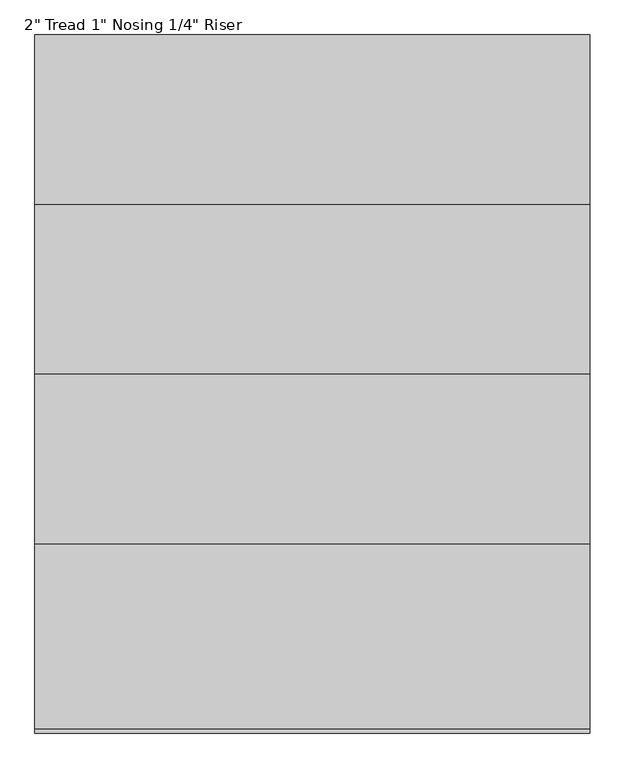
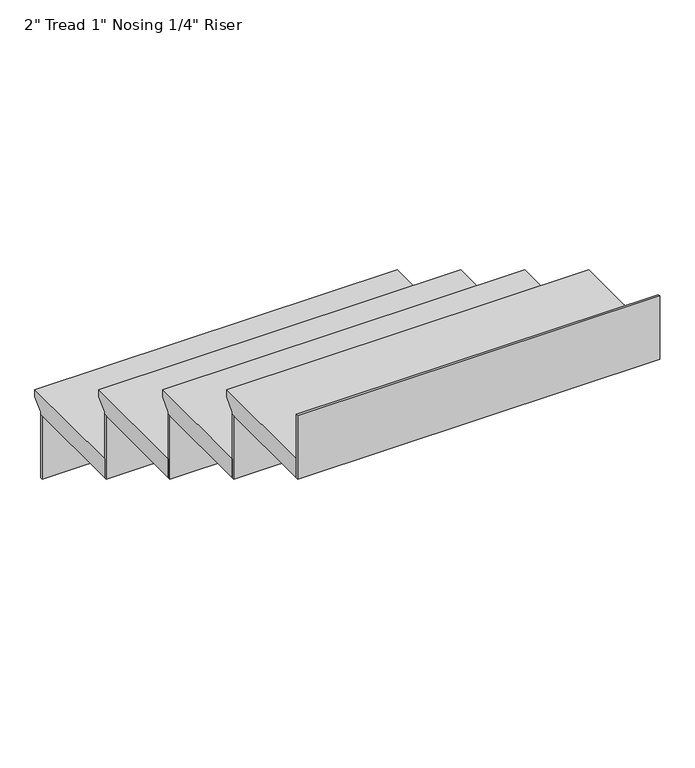
"""IFC4 building model written with IfcOpenShell, lengths in millimetres: stair flight geometry."""

from ifc_helpers import new_model, si_unit, frame, origin, place, context, project, spatial, polyline, outline, extrude, source, transform, mapped, element, save


def stair_flight_213872ae(model_context):
    return source(origin(), model_context, "Body", "SweptSolid", [
        extrude(outline(polyline([(22889.9216096, 27605.2839133), (23194.7216096, 27605.2839133), (23194.7216096, 27586.2339133), (23169.3216096, 27560.8339133), (23169.3216096, 27554.4839133), (22889.9216096, 27554.4839133), (22889.9216096, 27605.2839133)])), frame((-2398.2415084, 0.0, 0.0), z_axis=(1.0, 0.0, 0.0), x_axis=(0.0, 1.0, 0.0)), (0.0, 0.0, 1.0), 914.4),
        extrude(outline(polyline([(-2398.2415084, 23162.9716096), (-2398.2415084, 23169.3216096), (-1483.8415084, 23169.3216096), (-1483.8415084, 23162.9716096), (-2398.2415084, 23162.9716096)])), frame((0.0, 0.0, 27385.1505799), z_axis=(0.0, 0.0, 1.0), x_axis=(1.0, 0.0, 0.0)), (0.0, 0.0, 1.0), 169.3333333),
        extrude(outline(polyline([(-2398.2415084, 22883.5716096), (-2398.2415084, 22889.9216096), (-1483.8415084, 22889.9216096), (-1483.8415084, 22883.5716096), (-2398.2415084, 22883.5716096)])), frame((0.0, 0.0, 27554.4839133), z_axis=(0.0, 0.0, 1.0), x_axis=(1.0, 0.0, 0.0)), (0.0, 0.0, 1.0), 169.3333333),
        extrude(outline(polyline([(22610.5216096, 27774.6172466), (22915.3216096, 27774.6172466), (22915.3216096, 27755.5672466), (22889.9216096, 27730.1672466), (22889.9216096, 27723.8172466), (22610.5216096, 27723.8172466), (22610.5216096, 27774.6172466)])), frame((-2398.2415084, 0.0, 0.0), z_axis=(1.0, 0.0, 0.0), x_axis=(0.0, 1.0, 0.0)), (0.0, 0.0, 1.0), 914.4),
        extrude(outline(polyline([(-2398.2415084, 22604.1716096), (-2398.2415084, 22610.5216096), (-1483.8415084, 22610.5216096), (-1483.8415084, 22604.1716096), (-2398.2415084, 22604.1716096)])), frame((0.0, 0.0, 27723.8172466), z_axis=(0.0, 0.0, 1.0), x_axis=(1.0, 0.0, 0.0)), (0.0, 0.0, 1.0), 169.3333333),
        extrude(outline(polyline([(22331.1216096, 27943.9505799), (22635.9216096, 27943.9505799), (22635.9216096, 27924.9005799), (22610.5216096, 27899.5005799), (22610.5216096, 27893.1505799), (22331.1216096, 27893.1505799), (22331.1216096, 27943.9505799)])), frame((-2398.2415084, 0.0, 0.0), z_axis=(1.0, 0.0, 0.0), x_axis=(0.0, 1.0, 0.0)), (0.0, 0.0, 1.0), 914.4),
        extrude(outline(polyline([(-2398.2415084, 22324.7716096), (-2398.2415084, 22331.1216096), (-1483.8415084, 22331.1216096), (-1483.8415084, 22324.7716096), (-2398.2415084, 22324.7716096)])), frame((0.0, 0.0, 27893.1505799), z_axis=(0.0, 0.0, 1.0), x_axis=(1.0, 0.0, 0.0)), (0.0, 0.0, 1.0), 169.3333333),
        extrude(outline(polyline([(-2398.2415084, 22045.3716096), (-2398.2415084, 22051.7216096), (-1483.8415084, 22051.7216096), (-1483.8415084, 22045.3716096), (-2398.2415084, 22045.3716096)])), frame((0.0, 0.0, 28062.4839133), z_axis=(0.0, 0.0, 1.0), x_axis=(1.0, 0.0, 0.0)), (0.0, 0.0, 1.0), 169.3333333),
        extrude(outline(polyline([(22051.7216096, 28113.2839133), (22356.5216096, 28113.2839133), (22356.5216096, 28094.2339133), (22331.1216096, 28068.8339133), (22331.1216096, 28062.4839133), (22051.7216096, 28062.4839133), (22051.7216096, 28113.2839133)])), frame((-2398.2415084, 0.0, 0.0), z_axis=(1.0, 0.0, 0.0), x_axis=(0.0, 1.0, 0.0)), (0.0, 0.0, 1.0), 914.4),
    ])


if __name__ == "__main__":
    model = new_model("IFC4")
    model_context = context("Model", 3, world=origin())
    ifc_project = project(units=[si_unit("LENGTHUNIT", "METRE", prefix="MILLI")], contexts=[model_context])
    site = spatial("IfcSite", under=ifc_project)
    building = spatial("IfcBuilding", under=site)
    placement = place(None, origin())
    stair_flight_shape = stair_flight_213872ae(model_context)
    element("IfcStairFlight", 1, ObjectType="2\" Tread 1\" Nosing 1/4\" Riser", at=placement, inside=building, context=model_context, shape_type="MappedRepresentation", body=[
        mapped(stair_flight_shape, transform((0.0, 0.0, 0.0), x_axis=(1.0, 0.0, 0.0), y_axis=(0.0, 1.0, 0.0), z_axis=(0.0, 0.0, 1.0))),
    ])
    save(model, "model.ifc")
